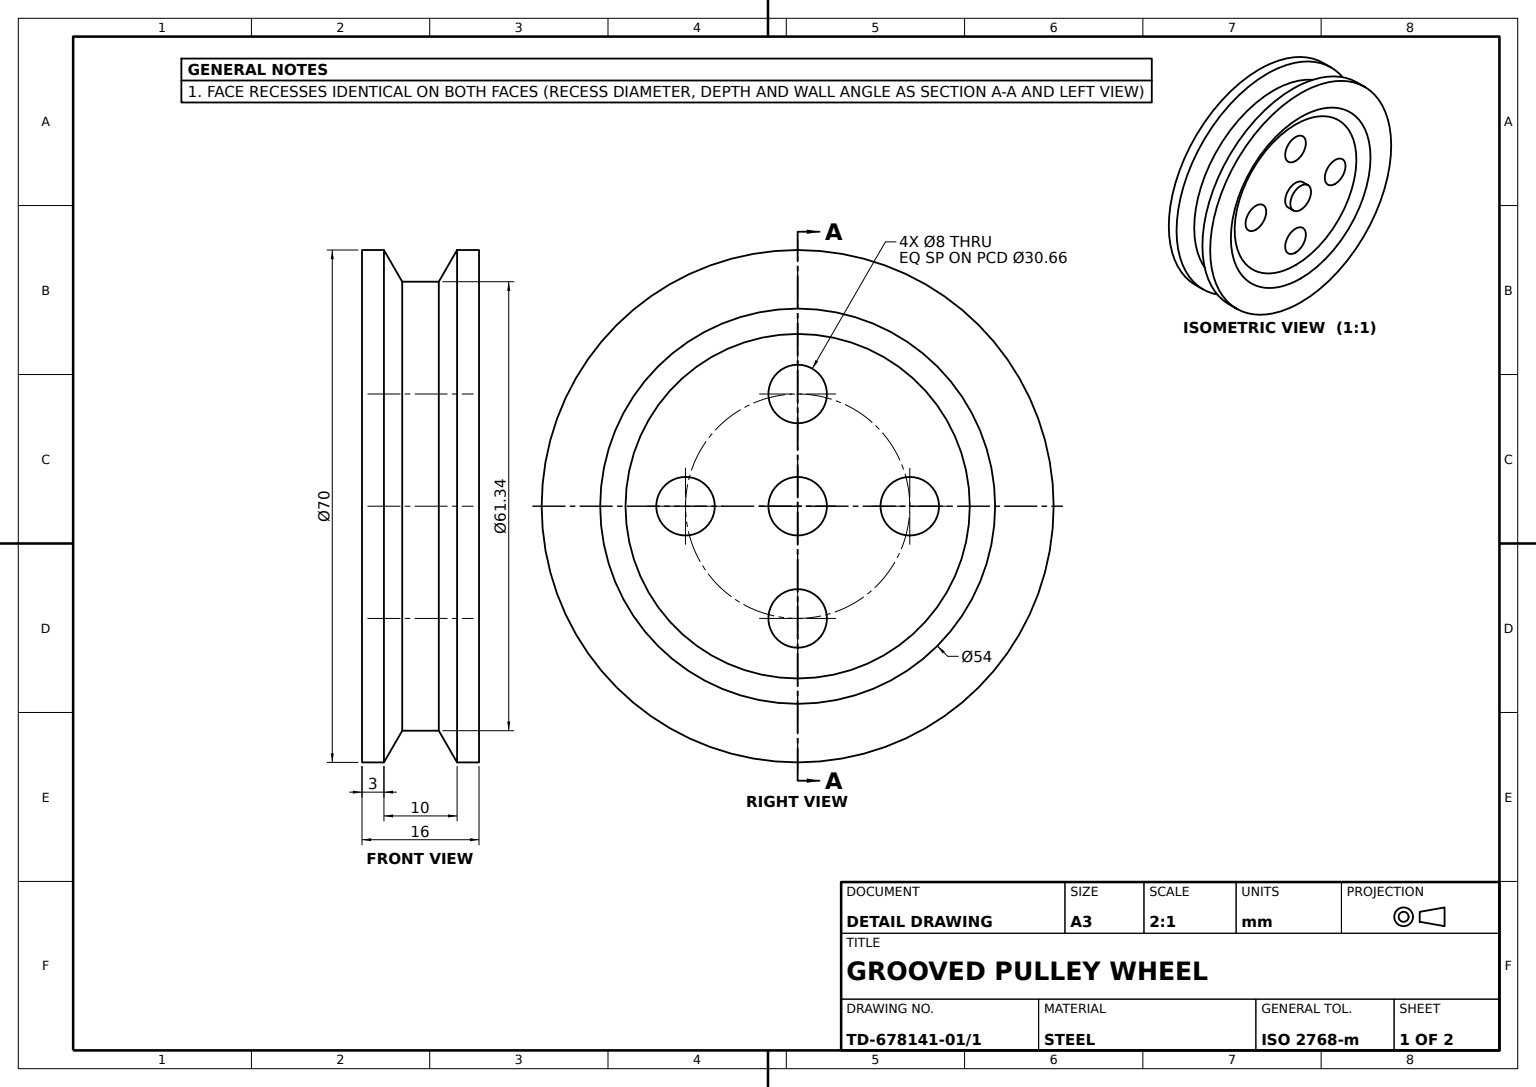
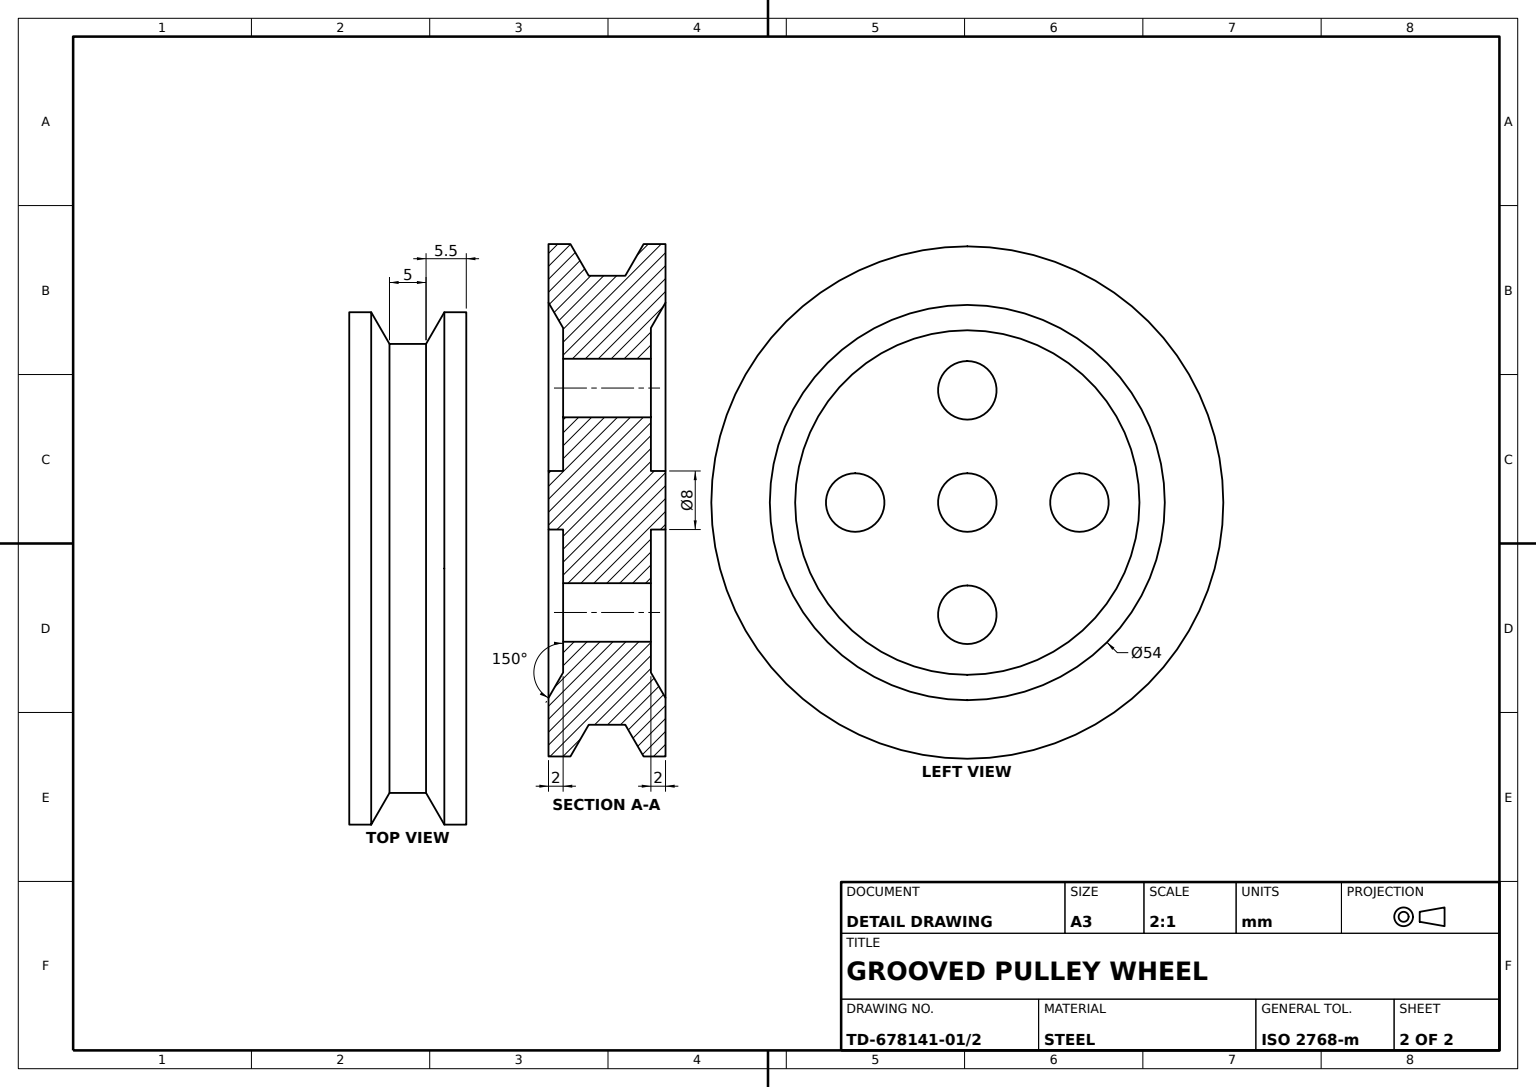
SolidWorks part; units mm, degrees
material "Plain Carbon Steel"
ref_plane "Front Plane" through (0, 0, 0) normal (0, 0, 1) x (1, 0, 0)
ref_plane "Top Plane" through (0, 0, 0) normal (0, 1, 0) x (1, 0, 0)
ref_plane "Right Plane" through (0, 0, 0) normal (1, 0, 0) x (0, 0, -1)
sketch "Pulley Profile Sketch" plane through (0, 0, 0) normal (0, 0, 1) x (1, 0, 0)
  line L0 (0, 17.9941) -> (0, 0) construction
  line L1 (0, 0) -> (-22.3566, 0) construction
  line L2 (8, 6) -> (-8, 6)
  line L3 (-8, 6) -> (-8, 10)
  line L4 (8, 6) -> (8, 10)
  line L5 (-8, 10) -> (-6, 10)
  line L6 (8, 10) -> (6, 10)
  line L7 (-6, 10) -> (-6, 29.5359)
  line L8 (6, 10) -> (6, 29.5359)
  line L9 (-6, 29.5359) -> (-8, 33)
  line L10 (6, 29.5359) -> (8, 33)
  line L11 (-8, 33) -> (-8, 41)
  line L12 (8, 33) -> (8, 41)
  line L13 (-8, 41) -> (-5, 41)
  line L14 (8, 41) -> (5, 41)
  line L15 (-5, 41) -> (-2.5, 36.6699)
  line L16 (5, 41) -> (2.5, 36.6699)
  line L17 (-2.5, 36.6699) -> (2.5, 36.6699)
  point P7 (0, 6)
  point P21 (8, 37)
  dimension "D1" = 16
  dimension "D2" = 35
  dimension "D3" = 6
  dimension "D4" = 10
  dimension "D5" = 12
  dimension "D6" = 150
  dimension "D7" = 8
  dimension "D8" = 5
  dimension "D9" = 5
  dimension "D10" = 16
  dimension "D11" = 4
revolve "Pulley Body" add sketch "Pulley Profile Sketch" angle 360 about L2
sketch "Hub Holes Sketch" plane through (-6, 0, 0) normal (-1, 0, 0) x (0, 0, 1)
  circle A0 centre (0, 6) radius 15.3296 construction
  circle A1 centre (0, 21.3296) radius 4
  circle A2 centre (-15.3296, 6) radius 4
  circle A3 centre (15.3296, 6) radius 4
  circle A4 centre (0, -9.3296) radius 4
  dimension "D1" = 30.6591
  dimension "D2" = 8
  dimension "D3" = 8
  dimension "D4" = 8
  dimension "D5" = 8
extrude "Hub Holes Ø8" cut sketch "Hub Holes Sketch" against normal through all
